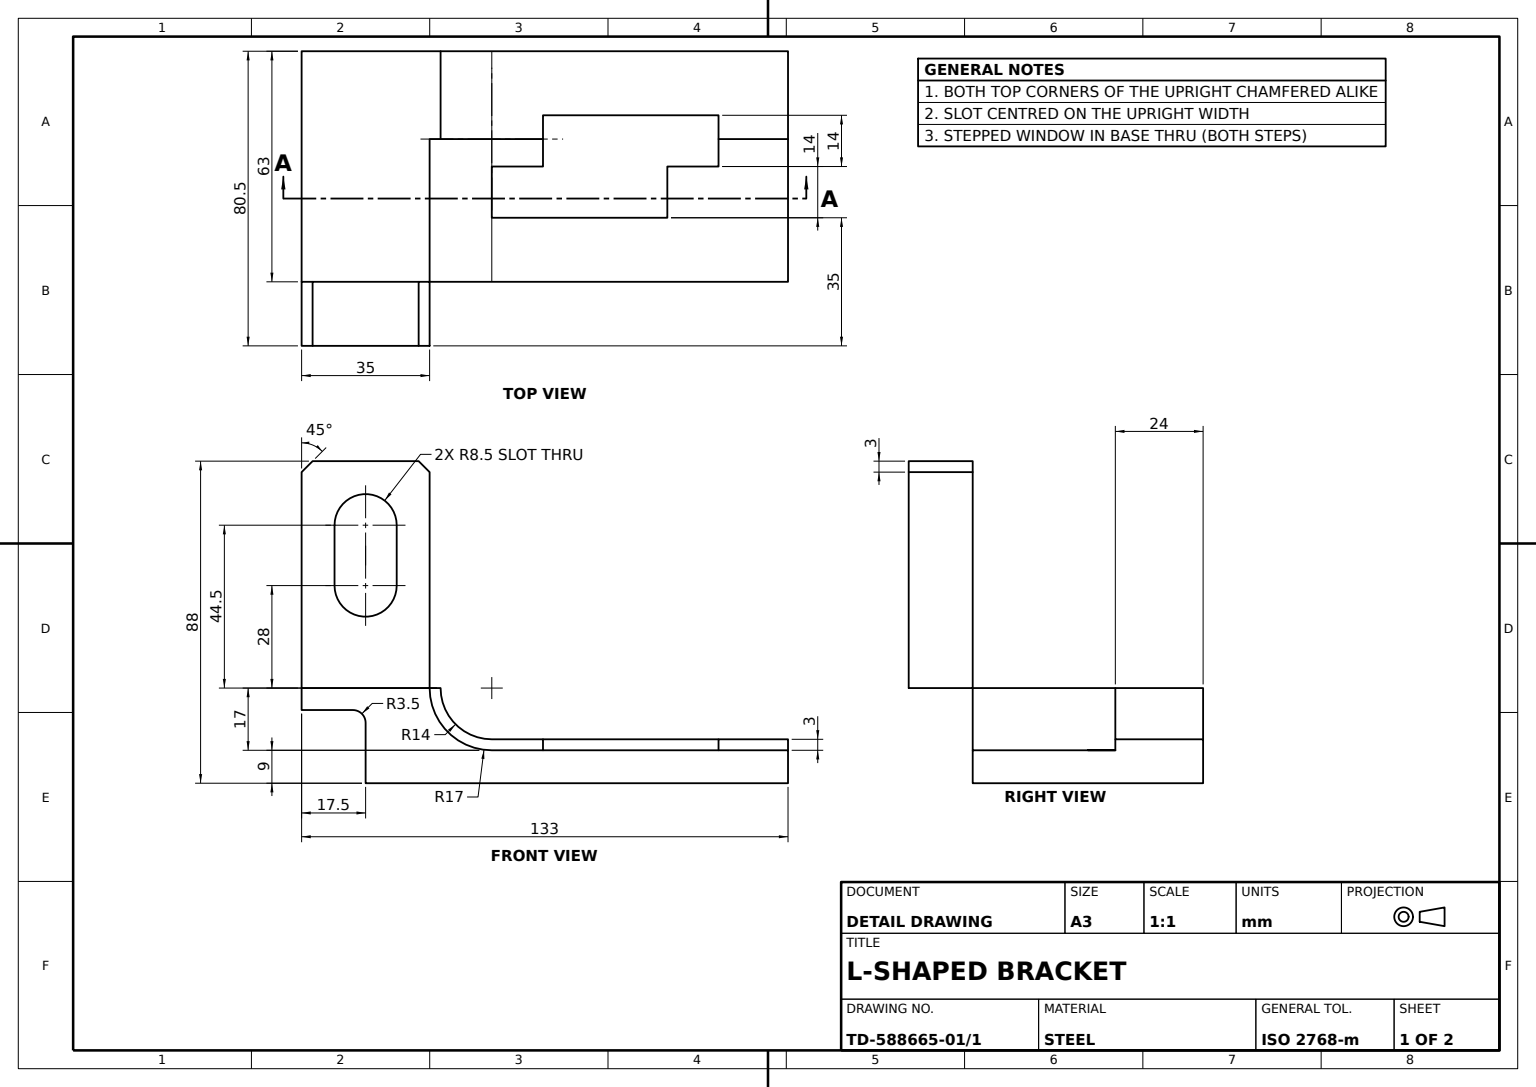
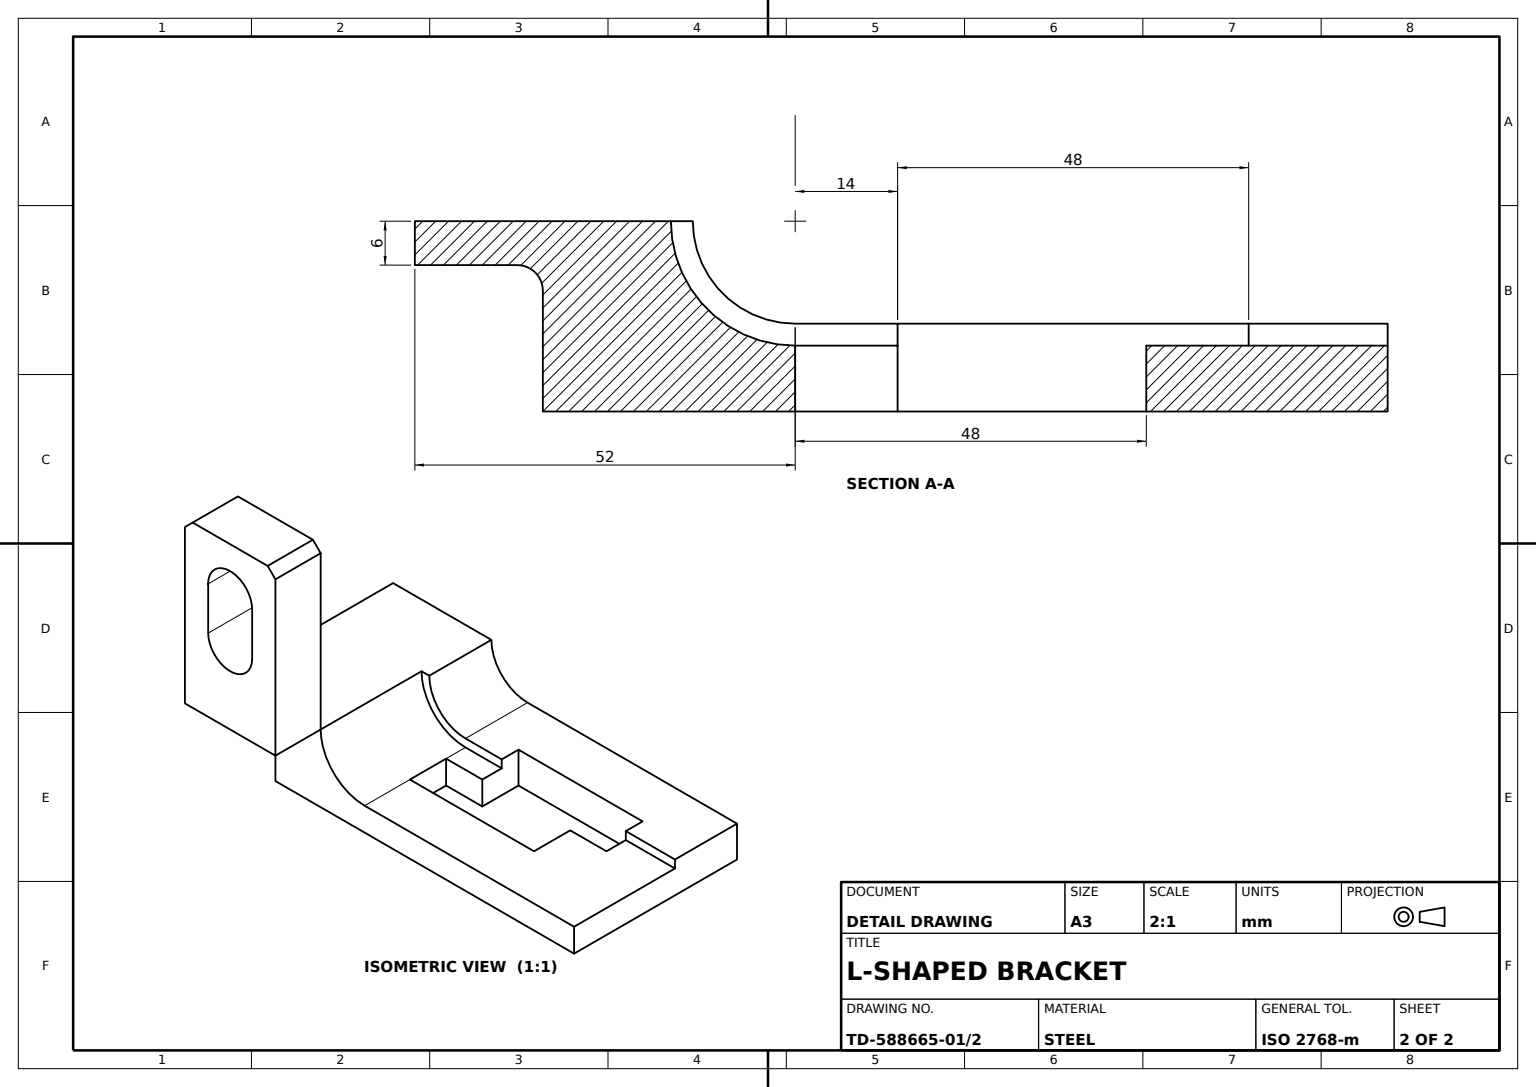
SolidWorks part; units mm, degrees
material "Plain Carbon Steel"
ref_plane "Front Plane" through (0, 0, 0) normal (0, 0, 1) x (1, 0, 0)
ref_plane "Top Plane" through (0, 0, 0) normal (0, 1, 0) x (1, 0, 0)
ref_plane "Right Plane" through (0, 0, 0) normal (1, 0, 0) x (0, 0, -1)
sketch "Base Profile Sketch" plane through (0, 0, 0) normal (0, 0, 1) x (1, 0, 0)
  line L0 (0, 0) -> (115.5, 0)
  line L2 (0, 0) -> (0, 16.5)
  line L3 (-3.5, 20) -> (-17.5, 20)
  line L8 (115.5, 9) -> (34.5, 9)
  line L11 (17.5, 26) -> (-17.5, 26)
  line L12 (-17.5, 26) -> (-17.5, 20)
  line L13 (115.5, 9) -> (115.5, 0)
  arc A0 (-3.5, 20) -> (0, 16.5) centre (-3.5, 16.5) cw
  arc A1 (17.5, 26) -> (34.5, 9) centre (34.5, 26) ccw
  dimension "D1" = 3.5
  dimension "D2" = 17
  dimension "D3" = 6
  dimension "D4" = 9
  dimension "D5" = 17.5
  dimension "D6" = 35
  dimension "D7" = 133
extrude "Base Plate" add sketch "Base Profile Sketch" along normal blind 63
sketch "Upright Block Sketch" plane through (0, 0, 63) normal (0, 0, 1) x (1, 0, 0)
  line L0 (0, 26) -> (17.5, 26)
  line L1 (17.5, 26) -> (-17.5, 26) construction
  line L2 (17.5, 26) -> (17.5, 54)
  line L3 (17.5, 70.5) -> (17.5, 85)
  line L4 (17.5, 54) -> (17.5, 70.5)
  line L8 (0, 88) -> (-14.5, 88)
  line L9 (0, 88) -> (14.5, 88)
  line L10 (14.5, 88) -> (17.5, 85)
  line L11 (-17.5, 26) -> (-17.5, 85)
  line L12 (-17.5, 85) -> (-14.5, 88)
  line L13 (0, 26) -> (-17.5, 26)
  dimension "D1" = 28
  dimension "D2" = 16.5
  dimension "D3" = 14.5
extrude "Upright Block" add sketch "Upright Block Sketch" along normal blind 17.5 separate body
sketch "Upright Slot Sketch" plane through (0, 0, 80.5) normal (0, 0, 1) x (1, 0, 0)
  line L0 (17.5, 26) -> (17.5, 85) construction
  line L1 (-17.5, 26) -> (17.5, 26) construction
  line L3 (-8.5, 70.5) -> (-8.5, 54)
  line L4 (8.5, 70.5) -> (8.5, 54)
  arc A0 (8.5, 70.5) -> (-8.5, 70.5) centre (0, 70.5) ccw
  arc A1 (-8.5, 54) -> (8.5, 54) centre (0, 54) ccw
  dimension "D1" = 8.5
  dimension "D2" = 17.5
  dimension "D3" = 28
  dimension "D4" = 44.5
extrude "Upright Obround Slot" cut sketch "Upright Slot Sketch" against normal blind 17.5
sketch "Stepped Window Sketch" plane through (0, 9, 0) normal (0, 1, 0) x (1, 0, 0)
  line L2 (96.5, -17.5) -> (48.5, -17.5)
  line L3 (96.5, -17.5) -> (96.5, -31.5)
  line L4 (96.5, -31.5) -> (82.5, -31.5)
  line L5 (82.5, -31.5) -> (82.5, -45.5)
  line L6 (82.5, -45.5) -> (34.5, -45.5)
  line L7 (34.5, -45.5) -> (34.5, -31.5)
  line L8 (34.5, -63) -> (34.5, 0) construction
  line L9 (48.5, -17.5) -> (48.5, -31.5)
  line L10 (48.5, -31.5) -> (34.5, -31.5)
  dimension "D1" = 14
  dimension "D2" = 48
extrude "Stepped Window Cut" cut sketch "Stepped Window Sketch" against normal blind 9
sketch "Raised Pad Sketch" plane through (0, 0, 0) normal (0, 0, -1) x (-1, 0, 0)
  line L1 (-34.5, 12) -> (-115.5, 12)
  line L2 (-115.5, 12) -> (-115.5, 9)
  line L3 (-115.5, 9) -> (-34.5, 9)
  line L4 (-17.5, 26) -> (-20.5, 26)
  arc A0 (-34.5, 12) -> (-20.5, 26) centre (-34.5, 26) ccw
  arc A1 (-34.5, 9) -> (-17.5, 26) centre (-34.5, 26) ccw
  dimension "D1" = 14
extrude "Raised Pad" add sketch "Raised Pad Sketch" against normal blind 24
sketch "Groove Sketch" plane through (0, 9, 0) normal (0, -1, 0) x (1, 0, 0)
  line L0 (48.5, 24) -> (96.5, 24)
  line L1 (96.5, 24) -> (96.5, 17.5)
  line L2 (96.5, 17.5) -> (48.5, 17.5)
  line L3 (48.5, 17.5) -> (48.5, 24)
extrude "Groove Cut 3mm" cut sketch "Groove Sketch" against normal blind 3
